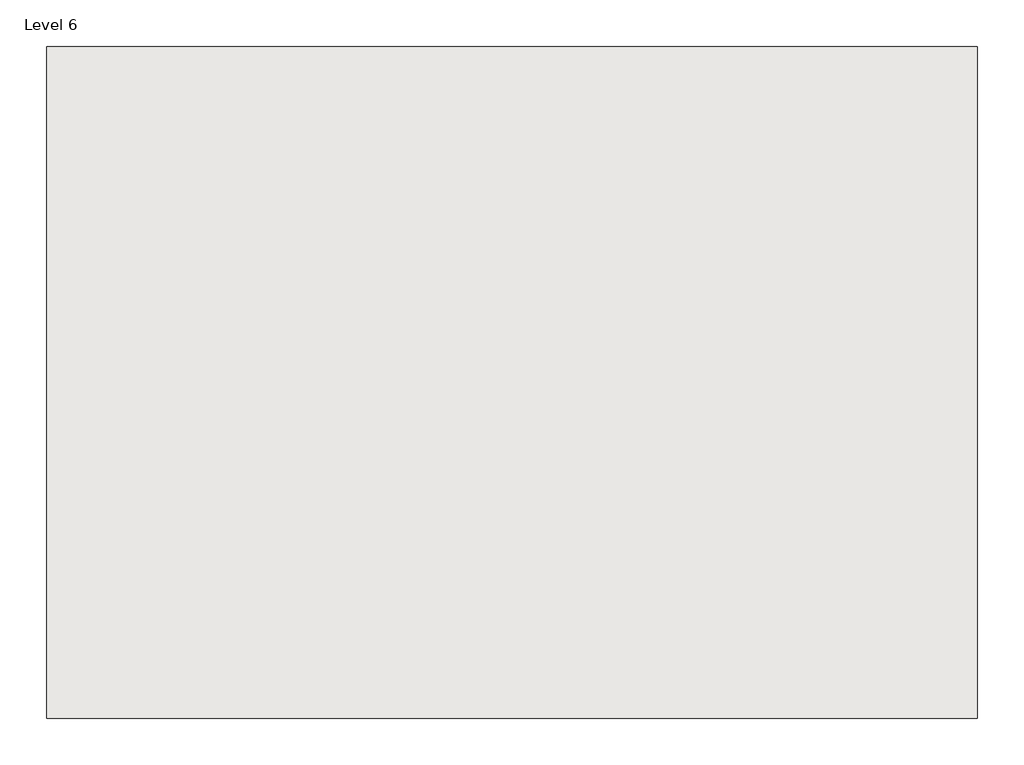
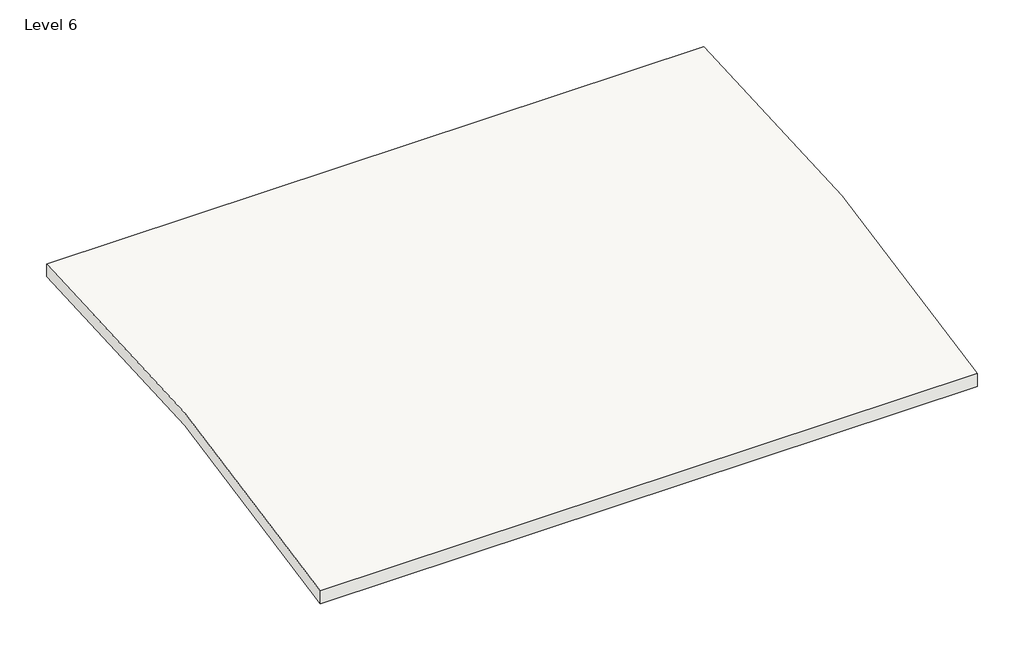
# One storey: 1 roof.
"""IFC4 building model written with IfcOpenShell, lengths in millimetres."""

from ifc_helpers import new_model, si_unit, point, frame, frame_2d, origin, place, context, project, spatial, polyline, circle_curve, trimmed, segment, composite_curve, outline, extrude, element, save

model = new_model("IFC4")

# Units and contexts
model_context = context("Model", 3, world=origin())
ifc_project = project(units=[si_unit("LENGTHUNIT", "METRE", prefix="MILLI")], contexts=[model_context])

# Site, building, storey
site = spatial("IfcSite", under=ifc_project)
building = spatial("IfcBuilding", under=site)
storey = spatial("IfcBuildingStorey", under=building, Name="Level 6", Elevation=7010.4)

# Roof
placement = place(None, origin())
element("IfcRoof", 1, ObjectType="Generic - 12\"", at=placement, inside=storey, context=model_context, shape_type="SweptSolid", body=[
    extrude(outline(composite_curve([segment(trimmed(circle_curve(frame_2d((-13694.3342361, -9875.5261928)), 12926.0560213), [point((-17068.9465604, 2602.2506896))], [point((-13438.6097562, 3048.0))], False, "CARTESIAN"), True, "CONTINUOUS"), segment(polyline([(-13438.6097562, 3048.0), (-13438.6097562, 2946.3799538)]), True, "CONTINUOUS"), segment(trimmed(circle_curve(frame_2d((-13694.3342361, -9875.5261928)), 12824.4560213), [point((-13438.6097562, 2946.3799538))], [point((-17068.9465604, 2496.9700752))], True, "CARTESIAN"), True, "CONTINUOUS"), segment(polyline([(-17068.9465604, 2496.9700752), (-17068.9465604, 2602.2506896)]), True, "CONTINUOUS")], self_intersect=False)), frame((-5651.4766939, 0.0, 0.0), z_axis=(1.0, 0.0, 0.0), x_axis=(0.0, 1.0, 0.0)), (0.0, 0.0, 1.0), 5029.2),
])

save(model, "model.ifc")

# Revit data of these elements
# Type "Generic - 12\""
#   Assembly Code = "B1020"
#   Layers, outside or top first: 0' - 4" no material (function 1)
# Element 1 (IfcRoof, "Generic - 12\"")
#   built-in parameter 1001710 = 33615
#   Phase Created = New Construction
#   Materials on its faces: "Default Roof", "3.GLASS"
# Materials
#   "Default Roof": colour RGB 88 101 114, transparency 0, Cost = 0
#   "3.GLASS": class "Generic", colour RGB 120 120 120, transparency 0, Cost = 0
